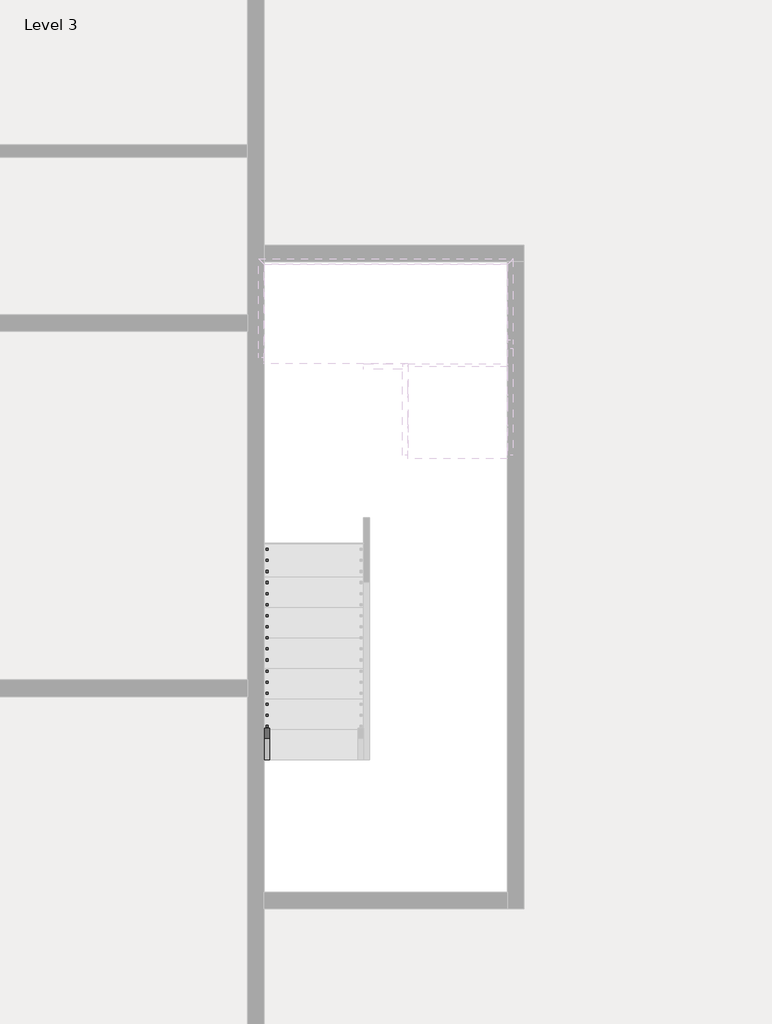
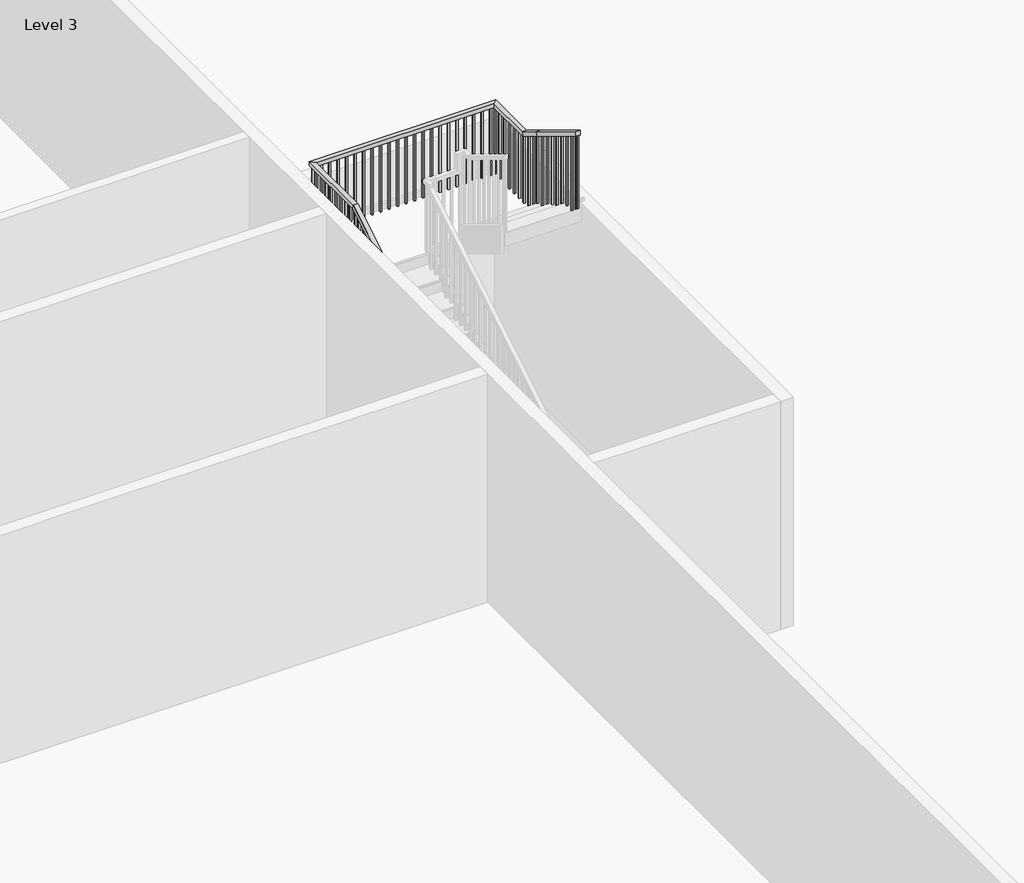
# One storey, part 6 of 8: 1 railing.
"""IFC4 building model written with IfcOpenShell, lengths in millimetres."""

from ifc_helpers import new_model, si_unit, frame, origin, place, context, project, spatial, polyline, outline, extrude, faceted_brep, element, save

model = new_model("IFC4")

# Units and contexts
model_context = context("Model", 3, world=origin())
ifc_project = project(units=[si_unit("LENGTHUNIT", "METRE", prefix="MILLI")], contexts=[model_context])

# Site, building, storey
site = spatial("IfcSite", under=ifc_project)
building = spatial("IfcBuilding", under=site)
storey = spatial("IfcBuildingStorey", under=building, Name="Level 3", Elevation=31330.6172466)

# Railing
placement = place(None, origin())
element("IfcRailing", 1, ObjectType="Handrail - Rectangular", at=placement, inside=storey, context=model_context, shape_type="SolidModel", body=[
    faceted_brep([(-3617.4415084, -23154.3851539, 32414.3505799), (-3617.4415084, -23154.3851539, 32354.9491197), (-3566.6415084, -23154.3851539, 32354.9491197), (-3566.6415084, -23154.3851539, 32414.3505799), (-3617.4415084, -19522.1851539, 34615.6839133), (-3617.4415084, -19507.9927445, 34564.8839133), (-3566.6415084, -19507.9927445, 34564.8839133), (-3566.6415084, -19522.1851539, 34615.6839133), (-3617.4415084, -18607.7851539, 34615.6839133), (-3617.4415084, -18607.7851539, 34564.8839133), (-3566.6415084, -18658.5851539, 34564.8839133), (-3566.6415084, -18658.5851539, 34615.6839133), (-1382.2415084, -18607.7851539, 34615.6839133), (-1382.2415084, -18607.7851539, 34564.8839133), (-1433.0415084, -18658.5851539, 34564.8839133), (-1433.0415084, -18658.5851539, 34615.6839133), (-1382.2415084, -19242.7851539, 34615.6839133), (-1382.2415084, -19256.9775633, 34564.8839133), (-1433.0415084, -19256.9775633, 34564.8839133), (-1433.0415084, -19242.7851539, 34615.6839133), (-1382.2415084, -19522.1851539, 34785.0172466), (-1382.2415084, -19548.5148811, 34741.5731968), (-1433.0415084, -19548.5148811, 34741.5731968), (-1433.0415084, -19522.1851539, 34785.0172466), (-1382.2415084, -20360.3851539, 35293.0172466), (-1433.0415084, -20360.3851539, 35293.0172466), (-1433.0415084, -20360.3851539, 35233.6157863), (-1382.2415084, -20360.3851539, 35233.6157863)], [[[0, 1, 2, 3]], [[1, 0, 4, 5]], [[2, 1, 5, 6]], [[3, 2, 6, 7]], [[0, 3, 7, 4]], [[5, 4, 8, 9]], [[6, 5, 9, 10]], [[7, 6, 10, 11]], [[4, 7, 11, 8]], [[9, 8, 12, 13]], [[10, 9, 13, 14]], [[11, 10, 14, 15]], [[8, 11, 15, 12]], [[13, 12, 16, 17]], [[14, 13, 17, 18]], [[15, 14, 18, 19]], [[12, 15, 19, 16]], [[17, 16, 20, 21]], [[18, 17, 21, 22]], [[19, 18, 22, 23]], [[16, 19, 23, 20]], [[24, 25, 26, 27]], [[21, 20, 24, 27]], [[22, 21, 27, 26]], [[23, 22, 26, 25]], [[20, 23, 25, 24]]]),
    extrude(outline(polyline([(-20325.4601539, 35212.4491197), (-20325.4601539, 34209.2839133), (-20344.5101539, 34209.2839133), (-20344.5101539, 35223.9945742), (-20325.4601539, 35212.4491197)])), frame((-1417.1665084, 0.0, 0.0), z_axis=(1.0, 0.0, 0.0), x_axis=(0.0, 1.0, 0.0)), (0.0, 0.0, 1.0), 19.05),
    extrude(outline(polyline([(-20223.8601539, 35150.8733621), (-20223.8601539, 34209.2839133), (-20242.9101539, 34209.2839133), (-20242.9101539, 35162.4188166), (-20223.8601539, 35150.8733621)])), frame((-1417.1665084, 0.0, 0.0), z_axis=(1.0, 0.0, 0.0), x_axis=(0.0, 1.0, 0.0)), (0.0, 0.0, 1.0), 19.05),
    extrude(outline(polyline([(-20122.2601539, 35089.2976045), (-20122.2601539, 34209.2839133), (-20141.3101539, 34209.2839133), (-20141.3101539, 35100.8430591), (-20122.2601539, 35089.2976045)])), frame((-1417.1665084, 0.0, 0.0), z_axis=(1.0, 0.0, 0.0), x_axis=(0.0, 1.0, 0.0)), (0.0, 0.0, 1.0), 19.05),
    extrude(outline(polyline([(-20020.6601539, 35027.721847), (-20020.6601539, 34039.9505799), (-20039.7101539, 34039.9505799), (-20039.7101539, 35039.2673015), (-20020.6601539, 35027.721847)])), frame((-1417.1665084, 0.0, 0.0), z_axis=(1.0, 0.0, 0.0), x_axis=(0.0, 1.0, 0.0)), (0.0, 0.0, 1.0), 19.05),
    extrude(outline(polyline([(-19919.0601539, 34966.1460894), (-19919.0601539, 34039.9505799), (-19938.1101539, 34039.9505799), (-19938.1101539, 34977.6915439), (-19919.0601539, 34966.1460894)])), frame((-1417.1665084, 0.0, 0.0), z_axis=(1.0, 0.0, 0.0), x_axis=(0.0, 1.0, 0.0)), (0.0, 0.0, 1.0), 19.05),
    extrude(outline(polyline([(-19817.4601539, 34904.5703318), (-19817.4601539, 34039.9505799), (-19836.5101539, 34039.9505799), (-19836.5101539, 34916.1157863), (-19817.4601539, 34904.5703318)])), frame((-1417.1665084, 0.0, 0.0), z_axis=(1.0, 0.0, 0.0), x_axis=(0.0, 1.0, 0.0)), (0.0, 0.0, 1.0), 19.05),
    extrude(outline(polyline([(-19715.8601539, 34842.9945742), (-19715.8601539, 33870.6172466), (-19734.9101539, 33870.6172466), (-19734.9101539, 34854.5400288), (-19715.8601539, 34842.9945742)])), frame((-1417.1665084, 0.0, 0.0), z_axis=(1.0, 0.0, 0.0), x_axis=(0.0, 1.0, 0.0)), (0.0, 0.0, 1.0), 19.05),
    extrude(outline(polyline([(-19614.2601539, 34781.4188166), (-19614.2601539, 33870.6172466), (-19633.3101539, 33870.6172466), (-19633.3101539, 34792.9642712), (-19614.2601539, 34781.4188166)])), frame((-1417.1665084, 0.0, 0.0), z_axis=(1.0, 0.0, 0.0), x_axis=(0.0, 1.0, 0.0)), (0.0, 0.0, 1.0), 19.05),
    extrude(outline(polyline([(-19436.4601539, 34673.6612409), (-19436.4601539, 33701.2839133), (-19455.5101539, 33701.2839133), (-19455.5101539, 34685.2066954), (-19436.4601539, 34673.6612409)])), frame((-1417.1665084, 0.0, 0.0), z_axis=(1.0, 0.0, 0.0), x_axis=(0.0, 1.0, 0.0)), (0.0, 0.0, 1.0), 19.05),
    extrude(outline(polyline([(-19334.8601539, 34612.0854833), (-19334.8601539, 33701.2839133), (-19353.9101539, 33701.2839133), (-19353.9101539, 34623.6309379), (-19334.8601539, 34612.0854833)])), frame((-1417.1665084, 0.0, 0.0), z_axis=(1.0, 0.0, 0.0), x_axis=(0.0, 1.0, 0.0)), (0.0, 0.0, 1.0), 19.05),
    extrude(outline(polyline([(-1398.1165084, -19233.2601539), (-1398.1165084, -19252.3101539), (-1417.1665084, -19252.3101539), (-1417.1665084, -19233.2601539), (-1398.1165084, -19233.2601539)])), frame((0.0, 0.0, 33701.2839133), z_axis=(0.0, 0.0, 1.0), x_axis=(1.0, 0.0, 0.0)), (0.0, 0.0, 1.0), 863.6),
    extrude(outline(polyline([(-1398.1165084, -19131.6601539), (-1398.1165084, -19150.7101539), (-1417.1665084, -19150.7101539), (-1417.1665084, -19131.6601539), (-1398.1165084, -19131.6601539)])), frame((0.0, 0.0, 33701.2839133), z_axis=(0.0, 0.0, 1.0), x_axis=(1.0, 0.0, 0.0)), (0.0, 0.0, 1.0), 863.6),
    extrude(outline(polyline([(-1398.1165084, -19030.0601539), (-1398.1165084, -19049.1101539), (-1417.1665084, -19049.1101539), (-1417.1665084, -19030.0601539), (-1398.1165084, -19030.0601539)])), frame((0.0, 0.0, 33701.2839133), z_axis=(0.0, 0.0, 1.0), x_axis=(1.0, 0.0, 0.0)), (0.0, 0.0, 1.0), 863.6),
    extrude(outline(polyline([(-1398.1165084, -18928.4601539), (-1398.1165084, -18947.5101539), (-1417.1665084, -18947.5101539), (-1417.1665084, -18928.4601539), (-1398.1165084, -18928.4601539)])), frame((0.0, 0.0, 33701.2839133), z_axis=(0.0, 0.0, 1.0), x_axis=(1.0, 0.0, 0.0)), (0.0, 0.0, 1.0), 863.6),
    extrude(outline(polyline([(-1398.1165084, -18826.8601539), (-1398.1165084, -18845.9101539), (-1417.1665084, -18845.9101539), (-1417.1665084, -18826.8601539), (-1398.1165084, -18826.8601539)])), frame((0.0, 0.0, 33701.2839133), z_axis=(0.0, 0.0, 1.0), x_axis=(1.0, 0.0, 0.0)), (0.0, 0.0, 1.0), 863.6),
    extrude(outline(polyline([(-1398.1165084, -18725.2601539), (-1398.1165084, -18744.3101539), (-1417.1665084, -18744.3101539), (-1417.1665084, -18725.2601539), (-1398.1165084, -18725.2601539)])), frame((0.0, 0.0, 33701.2839133), z_axis=(0.0, 0.0, 1.0), x_axis=(1.0, 0.0, 0.0)), (0.0, 0.0, 1.0), 863.6),
    extrude(outline(polyline([(-1467.9665084, -18623.6601539), (-1448.9165084, -18623.6601539), (-1448.9165084, -18642.7101539), (-1467.9665084, -18642.7101539), (-1467.9665084, -18623.6601539)])), frame((0.0, 0.0, 33701.2839133), z_axis=(0.0, 0.0, 1.0), x_axis=(1.0, 0.0, 0.0)), (0.0, 0.0, 1.0), 863.6),
    extrude(outline(polyline([(-1569.5665084, -18623.6601539), (-1550.5165084, -18623.6601539), (-1550.5165084, -18642.7101539), (-1569.5665084, -18642.7101539), (-1569.5665084, -18623.6601539)])), frame((0.0, 0.0, 33701.2839133), z_axis=(0.0, 0.0, 1.0), x_axis=(1.0, 0.0, 0.0)), (0.0, 0.0, 1.0), 863.6),
    extrude(outline(polyline([(-1671.1665084, -18623.6601539), (-1652.1165084, -18623.6601539), (-1652.1165084, -18642.7101539), (-1671.1665084, -18642.7101539), (-1671.1665084, -18623.6601539)])), frame((0.0, 0.0, 33701.2839133), z_axis=(0.0, 0.0, 1.0), x_axis=(1.0, 0.0, 0.0)), (0.0, 0.0, 1.0), 863.6),
    extrude(outline(polyline([(-1772.7665084, -18623.6601539), (-1753.7165084, -18623.6601539), (-1753.7165084, -18642.7101539), (-1772.7665084, -18642.7101539), (-1772.7665084, -18623.6601539)])), frame((0.0, 0.0, 33701.2839133), z_axis=(0.0, 0.0, 1.0), x_axis=(1.0, 0.0, 0.0)), (0.0, 0.0, 1.0), 863.6),
    extrude(outline(polyline([(-1874.3665084, -18623.6601539), (-1855.3165084, -18623.6601539), (-1855.3165084, -18642.7101539), (-1874.3665084, -18642.7101539), (-1874.3665084, -18623.6601539)])), frame((0.0, 0.0, 33701.2839133), z_axis=(0.0, 0.0, 1.0), x_axis=(1.0, 0.0, 0.0)), (0.0, 0.0, 1.0), 863.6),
    extrude(outline(polyline([(-1975.9665084, -18623.6601539), (-1956.9165084, -18623.6601539), (-1956.9165084, -18642.7101539), (-1975.9665084, -18642.7101539), (-1975.9665084, -18623.6601539)])), frame((0.0, 0.0, 33701.2839133), z_axis=(0.0, 0.0, 1.0), x_axis=(1.0, 0.0, 0.0)), (0.0, 0.0, 1.0), 863.6),
    extrude(outline(polyline([(-2077.5665084, -18623.6601539), (-2058.5165084, -18623.6601539), (-2058.5165084, -18642.7101539), (-2077.5665084, -18642.7101539), (-2077.5665084, -18623.6601539)])), frame((0.0, 0.0, 33701.2839133), z_axis=(0.0, 0.0, 1.0), x_axis=(1.0, 0.0, 0.0)), (0.0, 0.0, 1.0), 863.6),
    extrude(outline(polyline([(-2179.1665084, -18623.6601539), (-2160.1165084, -18623.6601539), (-2160.1165084, -18642.7101539), (-2179.1665084, -18642.7101539), (-2179.1665084, -18623.6601539)])), frame((0.0, 0.0, 33701.2839133), z_axis=(0.0, 0.0, 1.0), x_axis=(1.0, 0.0, 0.0)), (0.0, 0.0, 1.0), 863.6),
    extrude(outline(polyline([(-2280.7665084, -18623.6601539), (-2261.7165084, -18623.6601539), (-2261.7165084, -18642.7101539), (-2280.7665084, -18642.7101539), (-2280.7665084, -18623.6601539)])), frame((0.0, 0.0, 33701.2839133), z_axis=(0.0, 0.0, 1.0), x_axis=(1.0, 0.0, 0.0)), (0.0, 0.0, 1.0), 863.6),
    extrude(outline(polyline([(-2382.3665084, -18623.6601539), (-2363.3165084, -18623.6601539), (-2363.3165084, -18642.7101539), (-2382.3665084, -18642.7101539), (-2382.3665084, -18623.6601539)])), frame((0.0, 0.0, 33701.2839133), z_axis=(0.0, 0.0, 1.0), x_axis=(1.0, 0.0, 0.0)), (0.0, 0.0, 1.0), 863.6),
    extrude(outline(polyline([(-2483.9665084, -18623.6601539), (-2464.9165084, -18623.6601539), (-2464.9165084, -18642.7101539), (-2483.9665084, -18642.7101539), (-2483.9665084, -18623.6601539)])), frame((0.0, 0.0, 33701.2839133), z_axis=(0.0, 0.0, 1.0), x_axis=(1.0, 0.0, 0.0)), (0.0, 0.0, 1.0), 863.6),
    extrude(outline(polyline([(-2585.5665084, -18623.6601539), (-2566.5165084, -18623.6601539), (-2566.5165084, -18642.7101539), (-2585.5665084, -18642.7101539), (-2585.5665084, -18623.6601539)])), frame((0.0, 0.0, 33701.2839133), z_axis=(0.0, 0.0, 1.0), x_axis=(1.0, 0.0, 0.0)), (0.0, 0.0, 1.0), 863.6),
    extrude(outline(polyline([(-2687.1665084, -18623.6601539), (-2668.1165084, -18623.6601539), (-2668.1165084, -18642.7101539), (-2687.1665084, -18642.7101539), (-2687.1665084, -18623.6601539)])), frame((0.0, 0.0, 33701.2839133), z_axis=(0.0, 0.0, 1.0), x_axis=(1.0, 0.0, 0.0)), (0.0, 0.0, 1.0), 863.6),
    extrude(outline(polyline([(-2788.7665084, -18623.6601539), (-2769.7165084, -18623.6601539), (-2769.7165084, -18642.7101539), (-2788.7665084, -18642.7101539), (-2788.7665084, -18623.6601539)])), frame((0.0, 0.0, 33701.2839133), z_axis=(0.0, 0.0, 1.0), x_axis=(1.0, 0.0, 0.0)), (0.0, 0.0, 1.0), 863.6),
    extrude(outline(polyline([(-2890.3665084, -18623.6601539), (-2871.3165084, -18623.6601539), (-2871.3165084, -18642.7101539), (-2890.3665084, -18642.7101539), (-2890.3665084, -18623.6601539)])), frame((0.0, 0.0, 33701.2839133), z_axis=(0.0, 0.0, 1.0), x_axis=(1.0, 0.0, 0.0)), (0.0, 0.0, 1.0), 863.6),
    extrude(outline(polyline([(-2991.9665084, -18623.6601539), (-2972.9165084, -18623.6601539), (-2972.9165084, -18642.7101539), (-2991.9665084, -18642.7101539), (-2991.9665084, -18623.6601539)])), frame((0.0, 0.0, 33701.2839133), z_axis=(0.0, 0.0, 1.0), x_axis=(1.0, 0.0, 0.0)), (0.0, 0.0, 1.0), 863.6),
    extrude(outline(polyline([(-3093.5665084, -18623.6601539), (-3074.5165084, -18623.6601539), (-3074.5165084, -18642.7101539), (-3093.5665084, -18642.7101539), (-3093.5665084, -18623.6601539)])), frame((0.0, 0.0, 33701.2839133), z_axis=(0.0, 0.0, 1.0), x_axis=(1.0, 0.0, 0.0)), (0.0, 0.0, 1.0), 863.6),
    extrude(outline(polyline([(-3195.1665084, -18623.6601539), (-3176.1165084, -18623.6601539), (-3176.1165084, -18642.7101539), (-3195.1665084, -18642.7101539), (-3195.1665084, -18623.6601539)])), frame((0.0, 0.0, 33701.2839133), z_axis=(0.0, 0.0, 1.0), x_axis=(1.0, 0.0, 0.0)), (0.0, 0.0, 1.0), 863.6),
    extrude(outline(polyline([(-3296.7665084, -18623.6601539), (-3277.7165084, -18623.6601539), (-3277.7165084, -18642.7101539), (-3296.7665084, -18642.7101539), (-3296.7665084, -18623.6601539)])), frame((0.0, 0.0, 33701.2839133), z_axis=(0.0, 0.0, 1.0), x_axis=(1.0, 0.0, 0.0)), (0.0, 0.0, 1.0), 863.6),
    extrude(outline(polyline([(-3398.3665084, -18623.6601539), (-3379.3165084, -18623.6601539), (-3379.3165084, -18642.7101539), (-3398.3665084, -18642.7101539), (-3398.3665084, -18623.6601539)])), frame((0.0, 0.0, 33701.2839133), z_axis=(0.0, 0.0, 1.0), x_axis=(1.0, 0.0, 0.0)), (0.0, 0.0, 1.0), 863.6),
    extrude(outline(polyline([(-3499.9665084, -18623.6601539), (-3480.9165084, -18623.6601539), (-3480.9165084, -18642.7101539), (-3499.9665084, -18642.7101539), (-3499.9665084, -18623.6601539)])), frame((0.0, 0.0, 33701.2839133), z_axis=(0.0, 0.0, 1.0), x_axis=(1.0, 0.0, 0.0)), (0.0, 0.0, 1.0), 863.6),
    extrude(outline(polyline([(-3601.5665084, -18718.9101539), (-3601.5665084, -18699.8601539), (-3582.5165084, -18699.8601539), (-3582.5165084, -18718.9101539), (-3601.5665084, -18718.9101539)])), frame((0.0, 0.0, 33701.2839133), z_axis=(0.0, 0.0, 1.0), x_axis=(1.0, 0.0, 0.0)), (0.0, 0.0, 1.0), 863.6),
    extrude(outline(polyline([(-3601.5665084, -18820.5101539), (-3601.5665084, -18801.4601539), (-3582.5165084, -18801.4601539), (-3582.5165084, -18820.5101539), (-3601.5665084, -18820.5101539)])), frame((0.0, 0.0, 33701.2839133), z_axis=(0.0, 0.0, 1.0), x_axis=(1.0, 0.0, 0.0)), (0.0, 0.0, 1.0), 863.6),
    extrude(outline(polyline([(-3601.5665084, -18922.1101539), (-3601.5665084, -18903.0601539), (-3582.5165084, -18903.0601539), (-3582.5165084, -18922.1101539), (-3601.5665084, -18922.1101539)])), frame((0.0, 0.0, 33701.2839133), z_axis=(0.0, 0.0, 1.0), x_axis=(1.0, 0.0, 0.0)), (0.0, 0.0, 1.0), 863.6),
    extrude(outline(polyline([(-3601.5665084, -19023.7101539), (-3601.5665084, -19004.6601539), (-3582.5165084, -19004.6601539), (-3582.5165084, -19023.7101539), (-3601.5665084, -19023.7101539)])), frame((0.0, 0.0, 33701.2839133), z_axis=(0.0, 0.0, 1.0), x_axis=(1.0, 0.0, 0.0)), (0.0, 0.0, 1.0), 863.6),
    extrude(outline(polyline([(-3601.5665084, -19125.3101539), (-3601.5665084, -19106.2601539), (-3582.5165084, -19106.2601539), (-3582.5165084, -19125.3101539), (-3601.5665084, -19125.3101539)])), frame((0.0, 0.0, 33701.2839133), z_axis=(0.0, 0.0, 1.0), x_axis=(1.0, 0.0, 0.0)), (0.0, 0.0, 1.0), 863.6),
    extrude(outline(polyline([(-3601.5665084, -19226.9101539), (-3601.5665084, -19207.8601539), (-3582.5165084, -19207.8601539), (-3582.5165084, -19226.9101539), (-3601.5665084, -19226.9101539)])), frame((0.0, 0.0, 33701.2839133), z_axis=(0.0, 0.0, 1.0), x_axis=(1.0, 0.0, 0.0)), (0.0, 0.0, 1.0), 863.6),
    extrude(outline(polyline([(-3601.5665084, -19328.5101539), (-3601.5665084, -19309.4601539), (-3582.5165084, -19309.4601539), (-3582.5165084, -19328.5101539), (-3601.5665084, -19328.5101539)])), frame((0.0, 0.0, 33701.2839133), z_axis=(0.0, 0.0, 1.0), x_axis=(1.0, 0.0, 0.0)), (0.0, 0.0, 1.0), 863.6),
    extrude(outline(polyline([(-3601.5665084, -19430.1101539), (-3601.5665084, -19411.0601539), (-3582.5165084, -19411.0601539), (-3582.5165084, -19430.1101539), (-3601.5665084, -19430.1101539)])), frame((0.0, 0.0, 33701.2839133), z_axis=(0.0, 0.0, 1.0), x_axis=(1.0, 0.0, 0.0)), (0.0, 0.0, 1.0), 863.6),
    extrude(outline(polyline([(-19588.8601539, 34515.8733621), (-19588.8601539, 33531.9505799), (-19607.9101539, 33531.9505799), (-19607.9101539, 34504.3279076), (-19588.8601539, 34515.8733621)])), frame((-3601.5665084, 0.0, 0.0), z_axis=(1.0, 0.0, 0.0), x_axis=(0.0, 1.0, 0.0)), (0.0, 0.0, 1.0), 19.05),
    extrude(outline(polyline([(-19690.4601539, 34454.2976045), (-19690.4601539, 33531.9505799), (-19709.5101539, 33531.9505799), (-19709.5101539, 34442.75215), (-19690.4601539, 34454.2976045)])), frame((-3601.5665084, 0.0, 0.0), z_axis=(1.0, 0.0, 0.0), x_axis=(0.0, 1.0, 0.0)), (0.0, 0.0, 1.0), 19.05),
    extrude(outline(polyline([(-19792.0601539, 34392.721847), (-19792.0601539, 33531.9505799), (-19811.1101539, 33531.9505799), (-19811.1101539, 34381.1763924), (-19792.0601539, 34392.721847)])), frame((-3601.5665084, 0.0, 0.0), z_axis=(1.0, 0.0, 0.0), x_axis=(0.0, 1.0, 0.0)), (0.0, 0.0, 1.0), 19.05),
    extrude(outline(polyline([(-19893.6601539, 34331.1460894), (-19893.6601539, 33362.6172466), (-19912.7101539, 33362.6172466), (-19912.7101539, 34319.6006348), (-19893.6601539, 34331.1460894)])), frame((-3601.5665084, 0.0, 0.0), z_axis=(1.0, 0.0, 0.0), x_axis=(0.0, 1.0, 0.0)), (0.0, 0.0, 1.0), 19.05),
    extrude(outline(polyline([(-19995.2601539, 34269.5703318), (-19995.2601539, 33362.6172466), (-20014.3101539, 33362.6172466), (-20014.3101539, 34258.0248773), (-19995.2601539, 34269.5703318)])), frame((-3601.5665084, 0.0, 0.0), z_axis=(1.0, 0.0, 0.0), x_axis=(0.0, 1.0, 0.0)), (0.0, 0.0, 1.0), 19.05),
    extrude(outline(polyline([(-20096.8601539, 34207.9945742), (-20096.8601539, 33193.2839133), (-20115.9101539, 33193.2839133), (-20115.9101539, 34196.4491197), (-20096.8601539, 34207.9945742)])), frame((-3601.5665084, 0.0, 0.0), z_axis=(1.0, 0.0, 0.0), x_axis=(0.0, 1.0, 0.0)), (0.0, 0.0, 1.0), 19.05),
    extrude(outline(polyline([(-20198.4601539, 34146.4188166), (-20198.4601539, 33193.2839133), (-20217.5101539, 33193.2839133), (-20217.5101539, 34134.8733621), (-20198.4601539, 34146.4188166)])), frame((-3601.5665084, 0.0, 0.0), z_axis=(1.0, 0.0, 0.0), x_axis=(0.0, 1.0, 0.0)), (0.0, 0.0, 1.0), 19.05),
    extrude(outline(polyline([(-20300.0601539, 34084.8430591), (-20300.0601539, 33193.2839133), (-20319.1101539, 33193.2839133), (-20319.1101539, 34073.2976045), (-20300.0601539, 34084.8430591)])), frame((-3601.5665084, 0.0, 0.0), z_axis=(1.0, 0.0, 0.0), x_axis=(0.0, 1.0, 0.0)), (0.0, 0.0, 1.0), 19.05),
    extrude(outline(polyline([(-20401.6601539, 34023.2673015), (-20401.6601539, 33023.9505799), (-20420.7101539, 33023.9505799), (-20420.7101539, 34011.721847), (-20401.6601539, 34023.2673015)])), frame((-3601.5665084, 0.0, 0.0), z_axis=(1.0, 0.0, 0.0), x_axis=(0.0, 1.0, 0.0)), (0.0, 0.0, 1.0), 19.05),
    extrude(outline(polyline([(-20503.2601539, 33961.6915439), (-20503.2601539, 33023.9505799), (-20522.3101539, 33023.9505799), (-20522.3101539, 33950.1460894), (-20503.2601539, 33961.6915439)])), frame((-3601.5665084, 0.0, 0.0), z_axis=(1.0, 0.0, 0.0), x_axis=(0.0, 1.0, 0.0)), (0.0, 0.0, 1.0), 19.05),
    extrude(outline(polyline([(-20604.8601539, 33900.1157863), (-20604.8601539, 33023.9505799), (-20623.9101539, 33023.9505799), (-20623.9101539, 33888.5703318), (-20604.8601539, 33900.1157863)])), frame((-3601.5665084, 0.0, 0.0), z_axis=(1.0, 0.0, 0.0), x_axis=(0.0, 1.0, 0.0)), (0.0, 0.0, 1.0), 19.05),
    extrude(outline(polyline([(-20706.4601539, 33838.5400288), (-20706.4601539, 32854.6172466), (-20725.5101539, 32854.6172466), (-20725.5101539, 33826.9945742), (-20706.4601539, 33838.5400288)])), frame((-3601.5665084, 0.0, 0.0), z_axis=(1.0, 0.0, 0.0), x_axis=(0.0, 1.0, 0.0)), (0.0, 0.0, 1.0), 19.05),
    extrude(outline(polyline([(-20808.0601539, 33776.9642712), (-20808.0601539, 32854.6172466), (-20827.1101539, 32854.6172466), (-20827.1101539, 33765.4188166), (-20808.0601539, 33776.9642712)])), frame((-3601.5665084, 0.0, 0.0), z_axis=(1.0, 0.0, 0.0), x_axis=(0.0, 1.0, 0.0)), (0.0, 0.0, 1.0), 19.05),
    extrude(outline(polyline([(-20909.6601539, 33715.3885136), (-20909.6601539, 32854.6172466), (-20928.7101539, 32854.6172466), (-20928.7101539, 33703.8430591), (-20909.6601539, 33715.3885136)])), frame((-3601.5665084, 0.0, 0.0), z_axis=(1.0, 0.0, 0.0), x_axis=(0.0, 1.0, 0.0)), (0.0, 0.0, 1.0), 19.05),
    extrude(outline(polyline([(-21011.2601539, 33653.812756), (-21011.2601539, 32685.2839133), (-21030.3101539, 32685.2839133), (-21030.3101539, 33642.2673015), (-21011.2601539, 33653.812756)])), frame((-3601.5665084, 0.0, 0.0), z_axis=(1.0, 0.0, 0.0), x_axis=(0.0, 1.0, 0.0)), (0.0, 0.0, 1.0), 19.05),
    extrude(outline(polyline([(-21112.8601539, 33592.2369985), (-21112.8601539, 32685.2839133), (-21131.9101539, 32685.2839133), (-21131.9101539, 33580.6915439), (-21112.8601539, 33592.2369985)])), frame((-3601.5665084, 0.0, 0.0), z_axis=(1.0, 0.0, 0.0), x_axis=(0.0, 1.0, 0.0)), (0.0, 0.0, 1.0), 19.05),
    extrude(outline(polyline([(-21214.4601539, 33530.6612409), (-21214.4601539, 32515.9505799), (-21233.5101539, 32515.9505799), (-21233.5101539, 33519.1157863), (-21214.4601539, 33530.6612409)])), frame((-3601.5665084, 0.0, 0.0), z_axis=(1.0, 0.0, 0.0), x_axis=(0.0, 1.0, 0.0)), (0.0, 0.0, 1.0), 19.05),
    extrude(outline(polyline([(-21316.0601539, 33469.0854833), (-21316.0601539, 32515.9505799), (-21335.1101539, 32515.9505799), (-21335.1101539, 33457.5400288), (-21316.0601539, 33469.0854833)])), frame((-3601.5665084, 0.0, 0.0), z_axis=(1.0, 0.0, 0.0), x_axis=(0.0, 1.0, 0.0)), (0.0, 0.0, 1.0), 19.05),
    extrude(outline(polyline([(-21417.6601539, 33407.5097257), (-21417.6601539, 32515.9505799), (-21436.7101539, 32515.9505799), (-21436.7101539, 33395.9642712), (-21417.6601539, 33407.5097257)])), frame((-3601.5665084, 0.0, 0.0), z_axis=(1.0, 0.0, 0.0), x_axis=(0.0, 1.0, 0.0)), (0.0, 0.0, 1.0), 19.05),
    extrude(outline(polyline([(-21519.2601539, 33345.9339682), (-21519.2601539, 32346.6172466), (-21538.3101539, 32346.6172466), (-21538.3101539, 33334.3885136), (-21519.2601539, 33345.9339682)])), frame((-3601.5665084, 0.0, 0.0), z_axis=(1.0, 0.0, 0.0), x_axis=(0.0, 1.0, 0.0)), (0.0, 0.0, 1.0), 19.05),
    extrude(outline(polyline([(-21620.8601539, 33284.3582106), (-21620.8601539, 32346.6172466), (-21639.9101539, 32346.6172466), (-21639.9101539, 33272.812756), (-21620.8601539, 33284.3582106)])), frame((-3601.5665084, 0.0, 0.0), z_axis=(1.0, 0.0, 0.0), x_axis=(0.0, 1.0, 0.0)), (0.0, 0.0, 1.0), 19.05),
    extrude(outline(polyline([(-21722.4601539, 33222.782453), (-21722.4601539, 32346.6172466), (-21741.5101539, 32346.6172466), (-21741.5101539, 33211.2369985), (-21722.4601539, 33222.782453)])), frame((-3601.5665084, 0.0, 0.0), z_axis=(1.0, 0.0, 0.0), x_axis=(0.0, 1.0, 0.0)), (0.0, 0.0, 1.0), 19.05),
    extrude(outline(polyline([(-21824.0601539, 33161.2066954), (-21824.0601539, 32177.2839133), (-21843.1101539, 32177.2839133), (-21843.1101539, 33149.6612409), (-21824.0601539, 33161.2066954)])), frame((-3601.5665084, 0.0, 0.0), z_axis=(1.0, 0.0, 0.0), x_axis=(0.0, 1.0, 0.0)), (0.0, 0.0, 1.0), 19.05),
    extrude(outline(polyline([(-21925.6601539, 33099.6309379), (-21925.6601539, 32177.2839133), (-21944.7101539, 32177.2839133), (-21944.7101539, 33088.0854833), (-21925.6601539, 33099.6309379)])), frame((-3601.5665084, 0.0, 0.0), z_axis=(1.0, 0.0, 0.0), x_axis=(0.0, 1.0, 0.0)), (0.0, 0.0, 1.0), 19.05),
    extrude(outline(polyline([(-22027.2601539, 33038.0551803), (-22027.2601539, 32177.2839133), (-22046.3101539, 32177.2839133), (-22046.3101539, 33026.5097257), (-22027.2601539, 33038.0551803)])), frame((-3601.5665084, 0.0, 0.0), z_axis=(1.0, 0.0, 0.0), x_axis=(0.0, 1.0, 0.0)), (0.0, 0.0, 1.0), 19.05),
    extrude(outline(polyline([(-22128.8601539, 32976.4794227), (-22128.8601539, 32007.9505799), (-22147.9101539, 32007.9505799), (-22147.9101539, 32964.9339682), (-22128.8601539, 32976.4794227)])), frame((-3601.5665084, 0.0, 0.0), z_axis=(1.0, 0.0, 0.0), x_axis=(0.0, 1.0, 0.0)), (0.0, 0.0, 1.0), 19.05),
    extrude(outline(polyline([(-22230.4601539, 32914.9036651), (-22230.4601539, 32007.9505799), (-22249.5101539, 32007.9505799), (-22249.5101539, 32903.3582106), (-22230.4601539, 32914.9036651)])), frame((-3601.5665084, 0.0, 0.0), z_axis=(1.0, 0.0, 0.0), x_axis=(0.0, 1.0, 0.0)), (0.0, 0.0, 1.0), 19.05),
    extrude(outline(polyline([(-22332.0601539, 32853.3279076), (-22332.0601539, 31838.6172466), (-22351.1101539, 31838.6172466), (-22351.1101539, 32841.782453), (-22332.0601539, 32853.3279076)])), frame((-3601.5665084, 0.0, 0.0), z_axis=(1.0, 0.0, 0.0), x_axis=(0.0, 1.0, 0.0)), (0.0, 0.0, 1.0), 19.05),
    extrude(outline(polyline([(-22433.6601539, 32791.75215), (-22433.6601539, 31838.6172466), (-22452.7101539, 31838.6172466), (-22452.7101539, 32780.2066954), (-22433.6601539, 32791.75215)])), frame((-3601.5665084, 0.0, 0.0), z_axis=(1.0, 0.0, 0.0), x_axis=(0.0, 1.0, 0.0)), (0.0, 0.0, 1.0), 19.05),
    extrude(outline(polyline([(-22535.2601539, 32730.1763924), (-22535.2601539, 31838.6172466), (-22554.3101539, 31838.6172466), (-22554.3101539, 32718.6309379), (-22535.2601539, 32730.1763924)])), frame((-3601.5665084, 0.0, 0.0), z_axis=(1.0, 0.0, 0.0), x_axis=(0.0, 1.0, 0.0)), (0.0, 0.0, 1.0), 19.05),
    extrude(outline(polyline([(-22636.8601539, 32668.6006348), (-22636.8601539, 31669.2839133), (-22655.9101539, 31669.2839133), (-22655.9101539, 32657.0551803), (-22636.8601539, 32668.6006348)])), frame((-3601.5665084, 0.0, 0.0), z_axis=(1.0, 0.0, 0.0), x_axis=(0.0, 1.0, 0.0)), (0.0, 0.0, 1.0), 19.05),
    extrude(outline(polyline([(-22738.4601539, 32607.0248773), (-22738.4601539, 31669.2839133), (-22757.5101539, 31669.2839133), (-22757.5101539, 32595.4794227), (-22738.4601539, 32607.0248773)])), frame((-3601.5665084, 0.0, 0.0), z_axis=(1.0, 0.0, 0.0), x_axis=(0.0, 1.0, 0.0)), (0.0, 0.0, 1.0), 19.05),
    extrude(outline(polyline([(-22840.0601539, 32545.4491197), (-22840.0601539, 31669.2839133), (-22859.1101539, 31669.2839133), (-22859.1101539, 32533.9036651), (-22840.0601539, 32545.4491197)])), frame((-3601.5665084, 0.0, 0.0), z_axis=(1.0, 0.0, 0.0), x_axis=(0.0, 1.0, 0.0)), (0.0, 0.0, 1.0), 19.05),
    extrude(outline(polyline([(-22941.6601539, 32483.8733621), (-22941.6601539, 31499.9505799), (-22960.7101539, 31499.9505799), (-22960.7101539, 32472.3279076), (-22941.6601539, 32483.8733621)])), frame((-3601.5665084, 0.0, 0.0), z_axis=(1.0, 0.0, 0.0), x_axis=(0.0, 1.0, 0.0)), (0.0, 0.0, 1.0), 19.05),
    extrude(outline(polyline([(-23043.2601539, 32422.2976045), (-23043.2601539, 31499.9505799), (-23062.3101539, 31499.9505799), (-23062.3101539, 32410.75215), (-23043.2601539, 32422.2976045)])), frame((-3601.5665084, 0.0, 0.0), z_axis=(1.0, 0.0, 0.0), x_axis=(0.0, 1.0, 0.0)), (0.0, 0.0, 1.0), 19.05),
    extrude(outline(polyline([(-19512.6601539, 34719.8430591), (-19512.6601539, 33701.2839133), (-19531.7101539, 33701.2839133), (-19531.7101539, 34731.3885136), (-19512.6601539, 34719.8430591)])), frame((-1417.1665084, 0.0, 0.0), z_axis=(1.0, 0.0, 0.0), x_axis=(0.0, 1.0, 0.0)), (0.0, 0.0, 1.0), 19.05),
    extrude(outline(polyline([(-1417.1665084, -18623.6601539), (-1398.1165084, -18623.6601539), (-1398.1165084, -18642.7101539), (-1417.1665084, -18642.7101539), (-1417.1665084, -18623.6601539)])), frame((0.0, 0.0, 33701.2839133), z_axis=(0.0, 0.0, 1.0), x_axis=(1.0, 0.0, 0.0)), (0.0, 0.0, 1.0), 863.6),
    extrude(outline(polyline([(-3601.5665084, -18642.7101539), (-3601.5665084, -18623.6601539), (-3582.5165084, -18623.6601539), (-3582.5165084, -18642.7101539), (-3601.5665084, -18642.7101539)])), frame((0.0, 0.0, 33701.2839133), z_axis=(0.0, 0.0, 1.0), x_axis=(1.0, 0.0, 0.0)), (0.0, 0.0, 1.0), 863.6),
    extrude(outline(polyline([(-19512.6601539, 34562.0551803), (-19512.6601539, 33701.2839133), (-19531.7101539, 33701.2839133), (-19531.7101539, 34550.5097257), (-19512.6601539, 34562.0551803)])), frame((-3601.5665084, 0.0, 0.0), z_axis=(1.0, 0.0, 0.0), x_axis=(0.0, 1.0, 0.0)), (0.0, 0.0, 1.0), 19.05),
    extrude(outline(polyline([(-20341.3351539, 35222.0703318), (-20341.3351539, 34209.2839133), (-20360.3851539, 34209.2839133), (-20360.3851539, 35233.6157863), (-20341.3351539, 35222.0703318)])), frame((-1417.1665084, 0.0, 0.0), z_axis=(1.0, 0.0, 0.0), x_axis=(0.0, 1.0, 0.0)), (0.0, 0.0, 1.0), 19.05),
    extrude(outline(polyline([(-23135.3351539, 32366.4945742), (-23135.3351539, 31499.9505799), (-23154.3851539, 31499.9505799), (-23154.3851539, 32354.9491197), (-23135.3351539, 32366.4945742)])), frame((-3601.5665084, 0.0, 0.0), z_axis=(1.0, 0.0, 0.0), x_axis=(0.0, 1.0, 0.0)), (0.0, 0.0, 1.0), 19.05),
])

save(model, "model.ifc")

# Revit data of these elements
# Type "Handrail - Rectangular"
#   Assembly Code = "C2010400"
#   built-in parameter 1008612 = 0.0416667 (stored number, unit not read)
#   built-in parameter 1008611 = 0.0416667 (stored number, unit not read)
#   built-in parameter 1008609 = 0.333333 (stored number, unit not read)
#   built-in parameter 1008604 = 0.166667 (stored number, unit not read)
#   built-in parameter 1008603 = 0.166667 (stored number, unit not read)
#   Railing Height = 3' - 0"
#   built-in parameter 1008630 = 2
#   built-in parameter 1008610 = 2
#   built-in parameter 1008618 = Baluster - Square : 3/4"
# Element 1 (IfcRailing, "Handrail - Rectangular")
#   Phase Created = New Construction
